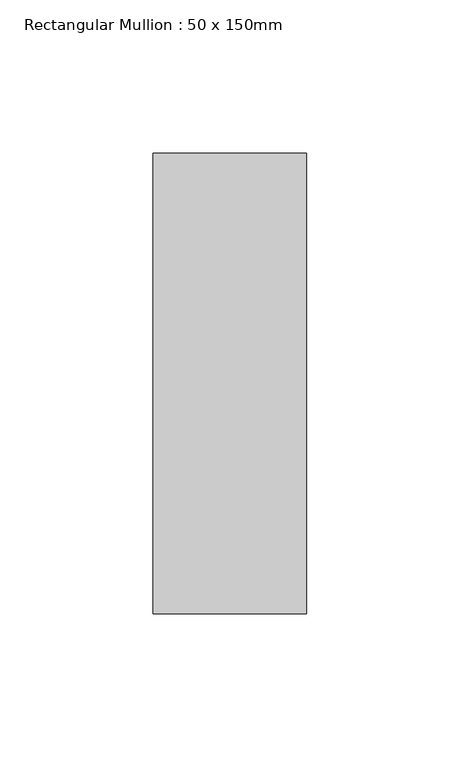
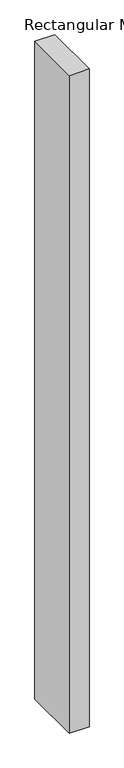
"""IFC4 building model written with IfcOpenShell, lengths in millimetres: member geometry, Rectangular Mullion : 50 x 150mm."""

from ifc_helpers import new_model, si_unit, frame, origin, place, context, project, spatial, polyline, outline, extrude, source, transform, mapped, element, save


def rectangular_mullion_50_x_150mm_86d49a4b(model_context):
    return source(origin(), model_context, "Body", "SweptSolid", [
        extrude(outline(polyline([(0.0, 75.0), (0.0, -75.0), (-50.0, -75.0), (-50.0, 75.0), (0.0, 75.0)])), frame((0.0, 0.0, -1755.0), z_axis=(0.0, 0.0, 1.0), x_axis=(1.0, 0.0, 0.0)), (0.0, 0.0, 1.0), 1755.0),
    ])


if __name__ == "__main__":
    model = new_model("IFC4")
    model_context = context("Model", 3, world=origin())
    ifc_project = project(units=[si_unit("LENGTHUNIT", "METRE", prefix="MILLI")], contexts=[model_context])
    site = spatial("IfcSite", under=ifc_project)
    building = spatial("IfcBuilding", under=site)
    placement = place(None, origin())
    rectangular_mullion_50_x_150mm_shape = rectangular_mullion_50_x_150mm_86d49a4b(model_context)
    element("IfcMember", 1, ObjectType="Rectangular Mullion : 50 x 150mm", at=placement, inside=building, context=model_context, shape_type="MappedRepresentation", body=[
        mapped(rectangular_mullion_50_x_150mm_shape, transform((0.0, 0.0, 0.0), x_axis=(1.0, 0.0, 0.0), y_axis=(0.0, 1.0, 0.0), z_axis=(0.0, 0.0, 1.0))),
    ])
    save(model, "model.ifc")

# Revit data of these elements
# Type "Rectangular Mullion : 50 x 150mm"
#   built-in parameter 1007304 = 0.492126 (stored number, unit not read)
#   built-in parameter 1007301 = 0.082021 (stored number, unit not read)
#   built-in parameter 1007300 = 0.082021 (stored number, unit not read)
# Element 1 (IfcMember, "Rectangular Mullion : 50 x 150mm")
#   Materials on its faces: "Aluminium"
# Materials
#   "Aluminium": class "Metal", colour RGB 247 247 247, transparency 0, Description = "Aluminium 6061", Cost = 0
